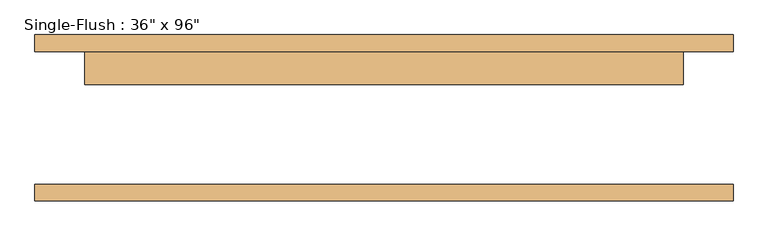
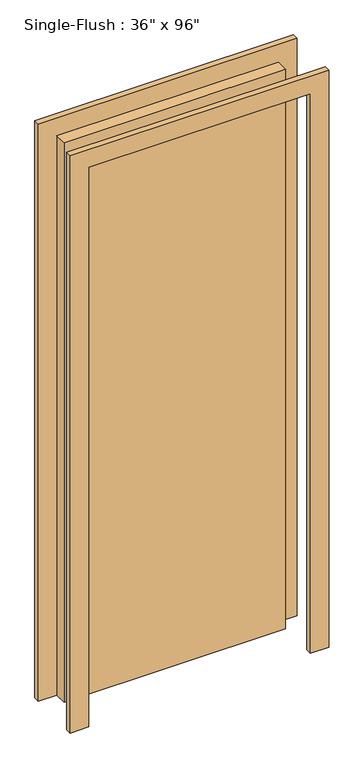
"""IFC4 building model written with IfcOpenShell, lengths in millimetres: door geometry."""

from ifc_helpers import new_model, si_unit, frame, origin, origin_with_axes, place, context, project, spatial, polyline, outline, extrude, source, transform, mapped, element, save


def door_f936a269(model_context):
    return source(origin(), model_context, "Body", "SweptSolid", [
        extrude(outline(polyline([(2514.6, -533.4), (0.0, -533.4), (0.0, -457.2), (2438.4, -457.2), (2438.4, 457.2), (0.0, 457.2), (0.0, 533.4), (2514.6, 533.4), (2514.6, -533.4)])), frame((0.0, 101.6, 0.0), z_axis=(0.0, 1.0, 0.0), x_axis=(0.0, 0.0, 1.0)), (0.0, 0.0, 1.0), 25.4),
        extrude(outline(polyline([(2514.6, 533.4), (2514.6, -533.4), (0.0, -533.4), (0.0, -457.2), (2438.4, -457.2), (2438.4, 457.2), (0.0, 457.2), (0.0, 533.4), (2514.6, 533.4)])), frame((0.0, -127.0, 0.0), z_axis=(0.0, 1.0, 0.0), x_axis=(0.0, 0.0, 1.0)), (0.0, 0.0, 1.0), 25.4),
        extrude(outline(polyline([(457.2, 50.8), (-457.2, 50.8), (-457.2, 101.6), (457.2, 101.6), (457.2, 50.8)])), origin_with_axes(), (0.0, 0.0, 1.0), 2438.4),
    ])


if __name__ == "__main__":
    model = new_model("IFC4")
    model_context = context("Model", 3, world=origin())
    ifc_project = project(units=[si_unit("LENGTHUNIT", "METRE", prefix="MILLI")], contexts=[model_context])
    site = spatial("IfcSite", under=ifc_project)
    building = spatial("IfcBuilding", under=site)
    placement = place(None, origin())
    door_shape = door_f936a269(model_context)
    element("IfcDoor", 1, ObjectType="Single-Flush : 36\" x 96\"", at=placement, inside=building, context=model_context, shape_type="MappedRepresentation", body=[
        mapped(door_shape, transform((0.0, 0.0, 0.0), x_axis=(1.0, 0.0, 0.0), y_axis=(0.0, 1.0, 0.0), z_axis=(0.0, 0.0, 1.0))),
    ])
    save(model, "model.ifc")

# Revit data of these elements
# Type "Single-Flush : 36\" x 96\""
#   Type Mark = "1"
#   Construction Type Id = "MDOOR"
#   Assembly Code = "C1020"
#   Analytic Construction = "Metal"
#   Thickness = 0' - 2"
#   Heat Transfer Coefficient (U) = 0.651978 BTU/(h·ft²·°F)
#   Height = 8' - 0"
#   Trim Projection Ext = 0' - 1"
#   Trim Projection Int = 0' - 1"
#   Trim Width = 0' - 3"
#   Width = 3' - 0"
#   Define Thermal Properties by = 1
#   Door Material = Glass, Clear Glazing
#   Frame Material = Iron, Ductile
#   Visual Light Transmittance = 0
#   Solar Heat Gain Coefficient = 0
#   Function = (empty or 0)
#   Wall Closure = (empty or 0)
# Element 1 (IfcDoor, "Single-Flush : 36\" x 96\"")
#   Materials on its faces: "Iron, Ductile", "Glass, Clear Glazing"
# Materials
#   "Glass, Clear Glazing": class "Glass", colour RGB 0 128 192, transparency 0.75, Description = "Clear glazing", Cost = 0
#   "Iron, Ductile": class "Metal", colour RGB 0 0 0, transparency 0, Description = "Ductile cast iron", Cost = 0
